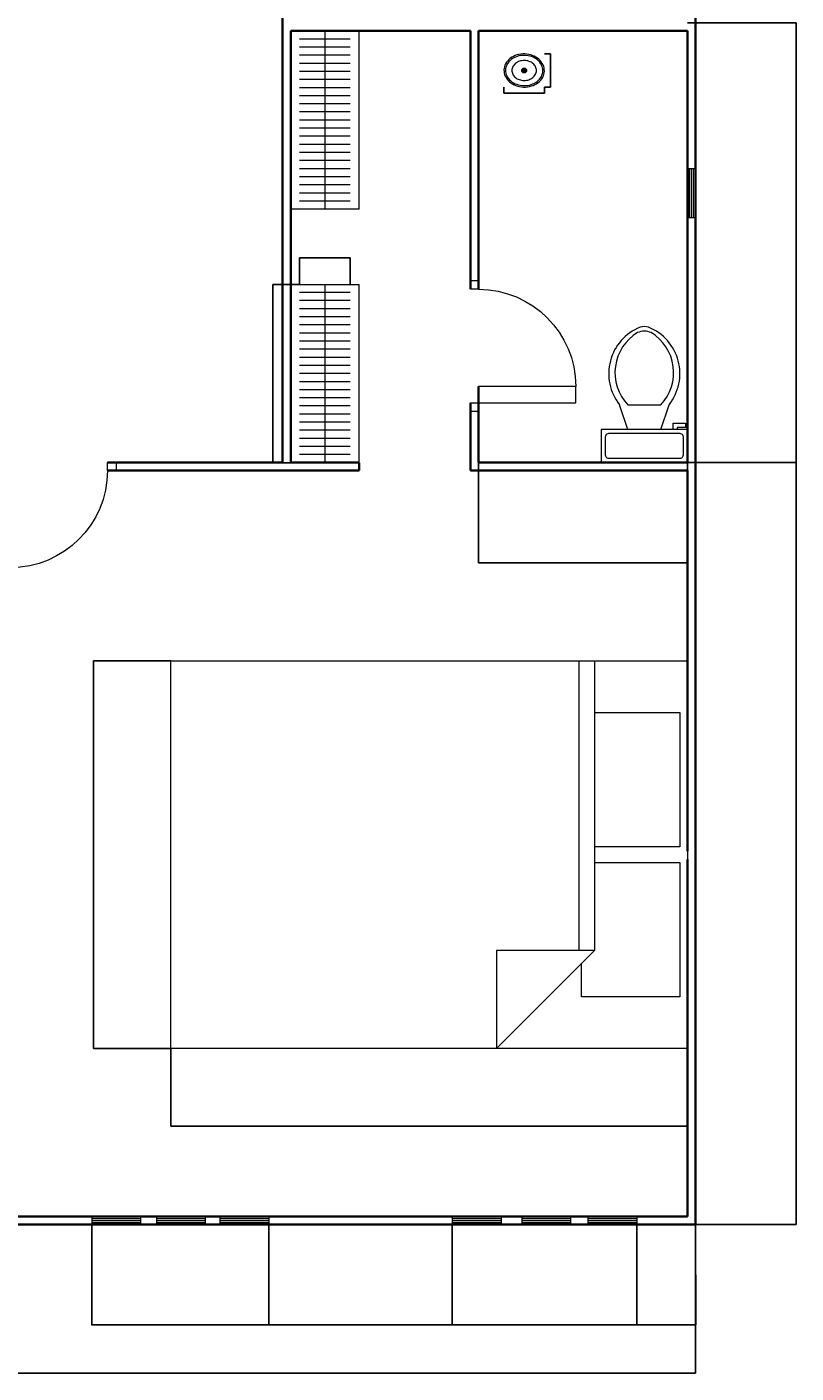
# Model space of a CAD drawing. Units: millimetres. Extents: x 1194 to 22780, y 83 to 13378.
# Tile 5 of 6: x 18030 to 22780, y 136 to 8443. Entities that reach past the tile are written whole.
import ezdxf

# ---------------------------------------------------------------- set-up
doc = ezdxf.new("R2010")
doc.units = ezdxf.units.MM
for name, color, linetype, lineweight in [('A-ANNO-DIMS', 2, 'Continuous', 18), ('A-DOOR', 3, 'Continuous', 18), ('A-FLOR-CASE', 8, 'Continuous', 13), ('A-FLOR-FIXT', 9, 'Continuous', 18), ('A-FURN', 8, 'Continuous', 18), ('A-GLAZ', 4, 'Continuous', 18), ('A-WALL', 7, 'Continuous', 35)]:
    doc.layers.add(name, color=color, linetype=linetype, lineweight=lineweight)
doc.styles.get("Standard").update_dxf_attribs({"font": 'arial.ttf'})
doc.dimstyles.get("Standard").update_dxf_attribs({"dimtxt": 0.18, "dimasz": 0.18, "dimexe": 0.18, "dimexo": 0.0625, "dimgap": 0.09, "dimtad": 0, "dimtih": 1, "dimtoh": 1, "dimdec": 4, "dimzin": 0, "dimdsep": 46, "dimtxsty": 'Standard', "dimcen": 0.09, "dimadec": 0, "dimazin": 0, "dimtfac": 1, "dimtdec": 4, "dimtofl": 0, "dimtmove": 0, "dimatfit": 3, "dimfxl": 1, "dimtolj": 1, "dimtzin": 0, "dimarcsym": 0})

# ---------------------------------------------------------------- blocks, each defined once
blk = doc.blocks.new('Bed - Queen')
for p, q in [((0, -80.00003), (0, 0)), ((0, 0), (59.99999, 0)), ((59.99999, 0), (59.99999, -80.00003)), ((7.99999, -1.2), (28.79998, -1.2)), ((7.99999, -14.4), (7.99999, -1.2)), ((28.79998, -1.2), (28.79998, -14.4)), ((31.19999, -1.2), (51.99999, -1.2)), ((31.19999, -14.4), (31.19999, -1.2)), ((51.99999, -1.2), (51.99999, -16.4)), ((0, -14.4), (44.8, -14.4)), ((59.99999, -29.6), (44.8, -14.4)), ((44.8, -14.4), (44.8, -29.6)), ((51.99999, -16.4), (46.79936, -16.4)), ((44.8, -16.8), (0, -16.8)), ((44.8, -29.6), (59.99999, -29.6)), ((59.99999, -80.00003), (0, -80.00003))]:
    blk.add_line(p, q)
blk = doc.blocks.new('Toilet - top')
for p, q in [((9.5, -6), (9.5, -2)), ((-10, -8.5), (-8, -8.5)), ((-10, -9.5), (-10, -8.5)), ((-7, -9.5), (-10, -9.5)), ((-8, -8.5), (-8, -8)), ((-7, -8), (-7, -9.5)), ((-4, -8), (-6, -14)), ((4, -8), (6, -14)), ((4, -14), (-4, -14))]:
    blk.add_line(p, q)
blk.add_lwpolyline([(10.5, -8), (10.5, 0), (-10.5, 0), (-10.5, -8)], close=True)
for points in [[(-9.5, -2), (-9.5, -6)], [(8.5, -1), (-8.5, -1)], [(-8.5, -7), (8.5, -7)]]:
    blk.add_lwpolyline(points)
for centre, radius, start, end in [((-8.62, -1.88), 0.884, 81.8699, 188.1301), ((8.62, -1.88), 0.884, 351.8699, 98.1301), ((-8.62, -6.12), 0.884, 171.8699, 278.1301), ((8.62, -6.12), 0.884, 261.8699, 8.1301), ((3.52, -21.58), 12.17, 141.4691, 247.9714), ((4.2, -21.82), 11.33, 136.3677, 238.9468), ((-3.52, -21.58), 12.17, 292.0284, 38.5307), ((-4.2, -21.82), 11.33, 301.053, 43.6321), ((0, -27.88), 4, 245.7318, 294.2682), ((0, -29), 4, 254.8605, 285.1395)]:
    blk.add_arc(centre, radius, start, end)
blk = doc.blocks.new('Sink - Oval top')
for p, q in [((-1, 0), (1, 0)), ((0, 1), (0, -1))]:
    blk.add_line(p, q)
for points in [[(-12.23, 0.39, 0.117634), (-11.46, -3.36, 0.104469), (-8.88, -6.8, 0.090016), (-5.08, -9.07, 0.08192), (-0.32, -10.02, 0.08192), (4.49, -9.38, 0.090016), (8.42, -7.36, 0.104469), (11.22, -4.09, 0.117634), (12.23, -0.39, 0.117634), (11.46, 3.36, 0.104469), (8.88, 6.8, 0.090016), (5.08, 9.07, 0.08192), (0.32, 10.02, 0.08192), (-4.49, 9.38, 0.090016), (-8.42, 7.36, 0.104469), (-11.22, 4.09, 0.117634)], [(-11.29, 0.16, 0.118622), (-10.52, -3.25, 0.104678), (-8.07, -6.36, 0.089562), (-4.54, -8.37, 0.081185), (-0.13, -9.15, 0.081185), (4.3, -8.49, 0.089562), (7.89, -6.58, 0.104678), (10.42, -3.55, 0.118622), (11.29, -0.16, 0.118622), (10.52, 3.25, 0.104678), (8.07, 6.36, 0.089562), (4.54, 8.37, 0.081185), (0.13, 9.15, 0.081185), (-4.3, 8.49, 0.089562), (-7.89, 6.58, 0.104678), (-10.42, 3.55, 0.118622)], [(-7.42, 0.08, 0.118283), (-6.91, -2.17, 0.104607), (-5.29, -4.21, 0.089718), (-2.97, -5.53, 0.081436), (-0.07, -6.04, 0.081436), (2.84, -5.59, 0.089718), (5.2, -4.33, 0.104607), (6.86, -2.32, 0.118283), (7.42, -0.08, 0.118283), (6.91, 2.17, 0.104607), (5.29, 4.21, 0.089718), (2.97, 5.53, 0.081436), (0.07, 6.04, 0.081436), (-2.84, 5.59, 0.089718), (-5.2, 4.33, 0.104607), (-6.86, 2.32, 0.118283)]]:
    blk.add_lwpolyline(points, format="xyb", close=True)
for radius in [1.5, 1]:
    blk.add_circle((0, 0), radius)
blk = doc.blocks.new('Window - Wood Frame 36 in. Wide plan')
for p, q in [((0, 6), (0, 0)), ((0, 4.5), (36, 4.5)), ((0, 3), (36, 3)), ((0, 1.5), (36, 1.5)), ((36, 6), (36, 0))]:
    blk.add_line(p, q)
blk = doc.blocks.new('DOOR-SWING-600')
for p, q in [((0, 0), (0, 600)), ((0, 600), (100, 600)), ((100, 600), (100, 0))]:
    blk.add_line(p, q)
blk.add_arc((100, 0), 600, 0, 90)
blk = doc.blocks.new('WARDROBE-RAIL-1100')
for p, q in [((156.2, 1100), (156.2, 0)), ((156.2, 1050), (0, 1050)), ((156.2, 1000), (0, 1000)), ((312.4, 1050), (156.2, 1050)), ((312.4, 1000), (156.2, 1000)), ((156.2, 950), (0, 950)), ((312.4, 950), (156.2, 950)), ((156.2, 900), (0, 900)), ((156.2, 850), (0, 850)), ((312.4, 900), (156.2, 900)), ((312.4, 850), (156.2, 850)), ((156.2, 800), (0, 800)), ((156.2, 750), (0, 750)), ((312.4, 800), (156.2, 800)), ((312.4, 750), (156.2, 750)), ((156.2, 700), (0, 700)), ((312.4, 700), (156.2, 700)), ((156.2, 650), (0, 650)), ((156.2, 600), (0, 600)), ((312.4, 650), (156.2, 650)), ((312.4, 600), (156.2, 600)), ((156.2, 550), (0, 550)), ((156.2, 500), (0, 500)), ((312.4, 550), (156.2, 550)), ((312.4, 500), (156.2, 500)), ((156.2, 450), (0, 450)), ((312.4, 450), (156.2, 450)), ((156.2, 400), (0, 400)), ((156.2, 350), (0, 350)), ((312.4, 400), (156.2, 400)), ((312.4, 350), (156.2, 350)), ((156.2, 300), (0, 300)), ((156.2, 250), (0, 250)), ((312.4, 300), (156.2, 300)), ((312.4, 250), (156.2, 250)), ((156.2, 200), (0, 200)), ((312.4, 200), (156.2, 200)), ((156.2, 150), (0, 150)), ((156.2, 100), (0, 100)), ((312.4, 150), (156.2, 150)), ((312.4, 100), (156.2, 100)), ((156.2, 50), (0, 50)), ((312.4, 50), (156.2, 50))]:
    blk.add_line(p, q)
blk = doc.blocks.new('*D23')
at = {"layer": 'A-ANNO-DIMS', "color": 0, "lineweight": -2, "transparency": 16777216}
for p, q in [((18919.4, 2138.4), (18919.4, 1659.8)), ((22109.2, 2138.4), (22109.2, 1659.8)), ((18919.6, 1659.9), (20513.7, 1659.9)), ((22109, 1659.9), (20515, 1659.9))]:
    blk.add_line(p, q, dxfattribs=at)
at = {"layer": 'A-ANNO-DIMS', "color": 0, "transparency": 16777216}
for points in [[(18919.6, 1660), (18919.6, 1659.9), (18919.4, 1659.9)], [(22109, 1660), (22109, 1659.9), (22109.2, 1659.9)]]:
    blk.add_solid(points, dxfattribs=at)
at = {"layer": 'Defpoints', "color": 0, "transparency": 16777216}
for p in [(18919.4, 2138.4), (22109.2, 2138.4), (22109.2, 1659.9)]:
    blk.add_point(p, dxfattribs=at)
at = {"layer": 'A-ANNO-DIMS', "color": 0, "transparency": 16777216, "insert": (20514.3, 1659.9), "char_height": 0.18, "attachment_point": 5}
blk.add_mtext('\\A1;BED 3190', dxfattribs=at)
blk = doc.blocks.new('*D24')
at = {"layer": 'A-ANNO-DIMS', "color": 0, "lineweight": -2, "transparency": 16777216}
for p, q in [((18919.3, 4530.8), (18440.7, 4530.8)), ((18440.9, 4530.6), (18440.9, 3334.8)), ((18440.9, 2138.6), (18440.9, 3334.4)), ((18919.3, 2138.4), (18440.7, 2138.4))]:
    blk.add_line(p, q, dxfattribs=at)
at = {"layer": 'A-ANNO-DIMS', "color": 0, "transparency": 16777216}
for points in [[(18440.9, 4530.6), (18441, 4530.6), (18440.9, 4530.8)], [(18440.9, 2138.6), (18441, 2138.6), (18440.9, 2138.4)]]:
    blk.add_solid(points, dxfattribs=at)
at = {"layer": 'Defpoints', "color": 0, "transparency": 16777216}
for p in [(18919.4, 4530.8), (18440.9, 2138.4), (18919.4, 2138.4)]:
    blk.add_point(p, dxfattribs=at)
at = {"layer": 'A-ANNO-DIMS', "color": 0, "transparency": 16777216, "insert": (18440.9, 3334.6), "char_height": 0.18, "attachment_point": 5}
blk.add_mtext('\\A1;2392', dxfattribs=at)
blk = doc.blocks.new('*D25')
at = {"layer": 'A-ANNO-DIMS', "color": 0, "lineweight": -2, "transparency": 16777216}
for p, q in [((20975.5, 8071.7), (20975.5, 8034)), ((21225.9, 8071.7), (21225.9, 8034)), ((20975.7, 8034.2), (21099.7, 8034.2)), ((21225.7, 8034.2), (21101.7, 8034.2))]:
    blk.add_line(p, q, dxfattribs=at)
at = {"layer": 'A-ANNO-DIMS', "color": 0, "transparency": 16777216}
for points in [[(20975.7, 8034.3), (20975.7, 8034.2), (20975.5, 8034.2)], [(21225.7, 8034.3), (21225.7, 8034.2), (21225.9, 8034.2)]]:
    blk.add_solid(points, dxfattribs=at)
at = {"layer": 'Defpoints', "color": 0, "transparency": 16777216}
for p in [(20975.5, 8071.8), (21225.9, 8071.8), (21225.9, 8034.2)]:
    blk.add_point(p, dxfattribs=at)
at = {"layer": 'A-ANNO-DIMS', "color": 0, "transparency": 16777216, "insert": (21100.7, 8034.2), "char_height": 0.18, "attachment_point": 5}
blk.add_mtext('\\A1;BASIN 250 TYP.', dxfattribs=at)
blk = doc.blocks.new('*D26')
at = {"layer": 'A-ANNO-DIMS', "color": 0, "lineweight": -2, "transparency": 16777216}
for p, q in [((21225.9, 8277.1), (21263.6, 8277.1)), ((21263.4, 8277), (21263.4, 8174.6)), ((21263.4, 8072), (21263.4, 8174.3)), ((21225.9, 8071.8), (21263.6, 8071.8))]:
    blk.add_line(p, q, dxfattribs=at)
at = {"layer": 'A-ANNO-DIMS', "color": 0, "transparency": 16777216}
for points in [[(21263.4, 8277), (21263.4, 8277), (21263.4, 8277.1)], [(21263.4, 8072), (21263.4, 8072), (21263.4, 8071.8)]]:
    blk.add_solid(points, dxfattribs=at)
at = {"layer": 'Defpoints', "color": 0, "transparency": 16777216}
for p in [(21225.9, 8277.1), (21263.4, 8277.1), (21225.9, 8071.8)]:
    blk.add_point(p, dxfattribs=at)
at = {"layer": 'A-ANNO-DIMS', "color": 0, "transparency": 16777216, "insert": (21263.4, 8174.5), "char_height": 0.18, "attachment_point": 5}
blk.add_mtext('\\A1;205 TYP.', dxfattribs=at)
blk = doc.blocks.new('*D41')
at = {"layer": 'A-ANNO-DIMS', "color": 0, "lineweight": -2, "transparency": 16777216}
for p, q in [((19714.1, 6854), (19549, 6854)), ((19549.2, 6853.8), (19549.2, 6304.2)), ((19549.2, 5754.2), (19549.2, 6303.8)), ((19714.1, 5754), (19549, 5754))]:
    blk.add_line(p, q, dxfattribs=at)
at = {"layer": 'A-ANNO-DIMS', "color": 0, "transparency": 16777216}
for points in [[(19549.2, 6853.8), (19549.2, 6853.8), (19549.2, 6854)], [(19549.2, 5754.2), (19549.2, 5754.2), (19549.2, 5754)]]:
    blk.add_solid(points, dxfattribs=at)
at = {"layer": 'Defpoints', "color": 0, "transparency": 16777216}
for p in [(19549.2, 6854), (19714.2, 6854), (19714.2, 5754)]:
    blk.add_point(p, dxfattribs=at)
at = {"layer": 'A-ANNO-DIMS', "color": 0, "transparency": 16777216, "insert": (19549.2, 6304), "char_height": 0.18, "attachment_point": 5}
blk.add_mtext('\\A1;CLOSET RAIL 1100 TYP.', dxfattribs=at)
blk = doc.blocks.new('*D42')
at = {"layer": 'A-ANNO-DIMS', "color": 0, "lineweight": -2, "transparency": 16777216}
for p, q in [((19714.2, 6854.1), (19714.2, 7019.2)), ((19714.4, 7019), (19869.8, 7019)), ((20026.4, 7019), (19871, 7019)), ((20026.6, 6854.1), (20026.6, 7019.2))]:
    blk.add_line(p, q, dxfattribs=at)
at = {"layer": 'A-ANNO-DIMS', "color": 0, "transparency": 16777216}
for points in [[(19714.4, 7019), (19714.4, 7019), (19714.2, 7019)], [(20026.4, 7019), (20026.4, 7019), (20026.6, 7019)]]:
    blk.add_solid(points, dxfattribs=at)
at = {"layer": 'Defpoints', "color": 0, "transparency": 16777216}
for p in [(20026.6, 7019), (19714.2, 6854), (20026.6, 6854)]:
    blk.add_point(p, dxfattribs=at)
at = {"layer": 'A-ANNO-DIMS', "color": 0, "transparency": 16777216, "insert": (19870.4, 7019), "char_height": 0.18, "attachment_point": 5}
blk.add_mtext('\\A1;312 TYP.', dxfattribs=at)
blk = doc.blocks.new('*D75')
at = {"layer": 'A-ANNO-DIMS', "color": 0, "lineweight": -2, "transparency": 16777216}
for p, q in [((22159.2, 1052.8), (22159.2, 135.6)), ((17634.2, 755.8), (17634.2, 135.6)), ((17634.4, 135.8), (19896.3, 135.8)), ((22159, 135.8), (19897.1, 135.8))]:
    blk.add_line(p, q, dxfattribs=at)
at = {"layer": 'A-ANNO-DIMS', "color": 0, "transparency": 16777216}
for points in [[(17634.4, 135.8), (17634.4, 135.8), (17634.2, 135.8)], [(22159, 135.8), (22159, 135.8), (22159.2, 135.8)]]:
    blk.add_solid(points, dxfattribs=at)
at = {"layer": 'Defpoints', "color": 0, "transparency": 16777216}
for p in [(22159.2, 1052.8), (17634.2, 755.8), (22159.2, 135.8)]:
    blk.add_point(p, dxfattribs=at)
at = {"layer": 'A-ANNO-DIMS', "color": 0, "transparency": 16777216, "insert": (19896.7, 135.8), "char_height": 0.18, "attachment_point": 5}
blk.add_mtext('\\A1;4525', dxfattribs=at)
blk = doc.blocks.new('*D76')
at = {"layer": 'A-ANNO-DIMS', "color": 0, "lineweight": -2, "transparency": 16777216}
for p, q in [((22109.3, 5755.8), (22779.4, 5755.8)), ((22779.2, 5755.6), (22779.2, 3404.5)), ((22779.2, 1053), (22779.2, 3404.1)), ((22159.3, 1052.8), (22779.4, 1052.8))]:
    blk.add_line(p, q, dxfattribs=at)
at = {"layer": 'A-ANNO-DIMS', "color": 0, "transparency": 16777216}
for points in [[(22779.2, 5755.6), (22779.2, 5755.6), (22779.2, 5755.8)], [(22779.2, 1053), (22779.2, 1053), (22779.2, 1052.8)]]:
    blk.add_solid(points, dxfattribs=at)
at = {"layer": 'Defpoints', "color": 0, "transparency": 16777216}
for p in [(22109.2, 5755.8), (22779.2, 5755.8), (22159.2, 1052.8)]:
    blk.add_point(p, dxfattribs=at)
at = {"layer": 'A-ANNO-DIMS', "color": 0, "transparency": 16777216, "insert": (22779.2, 3404.3), "char_height": 0.18, "attachment_point": 5}
blk.add_mtext('\\A1;4703', dxfattribs=at)
blk = doc.blocks.new('*D77')
at = {"layer": 'A-ANNO-DIMS', "color": 0, "lineweight": -2, "transparency": 16777216}
for p, q in [((22109.3, 8468.3), (22779.4, 8468.3)), ((22779.2, 8468.1), (22779.2, 7112.2)), ((22779.2, 5756), (22779.2, 7111.8)), ((22109.3, 5755.8), (22779.4, 5755.8))]:
    blk.add_line(p, q, dxfattribs=at)
at = {"layer": 'A-ANNO-DIMS', "color": 0, "transparency": 16777216}
for points in [[(22779.2, 8468.1), (22779.2, 8468.1), (22779.2, 8468.3)], [(22779.2, 5756), (22779.2, 5756), (22779.2, 5755.8)]]:
    blk.add_solid(points, dxfattribs=at)
at = {"layer": 'Defpoints', "color": 0, "transparency": 16777216}
for p in [(22109.2, 8468.3), (22779.2, 8468.3), (22109.2, 5755.8)]:
    blk.add_point(p, dxfattribs=at)
at = {"layer": 'A-ANNO-DIMS', "color": 0, "transparency": 16777216, "insert": (22779.2, 7112), "char_height": 0.18, "attachment_point": 5}
blk.add_mtext('\\A1;2712.5', dxfattribs=at)
blk = doc.blocks.new('*D85')
at = {"layer": 'A-ANNO-DIMS', "color": 0, "lineweight": -2, "transparency": 16777216}
for p, q in [((20818.9, 5755.7), (20818.9, 5135.6)), ((22109.2, 5755.7), (22109.2, 5135.6)), ((20819.1, 5135.8), (21463.6, 5135.8)), ((22109, 5135.8), (21464.5, 5135.8))]:
    blk.add_line(p, q, dxfattribs=at)
at = {"layer": 'A-ANNO-DIMS', "color": 0, "transparency": 16777216}
for points in [[(20819.1, 5135.8), (20819.1, 5135.7), (20818.9, 5135.8)], [(22109, 5135.8), (22109, 5135.7), (22109.2, 5135.8)]]:
    blk.add_solid(points, dxfattribs=at)
at = {"layer": 'Defpoints', "color": 0, "transparency": 16777216}
for p in [(20818.9, 5755.8), (22109.2, 5755.8), (20818.9, 5135.8)]:
    blk.add_point(p, dxfattribs=at)
at = {"layer": 'A-ANNO-DIMS', "color": 0, "transparency": 16777216, "insert": (21464.1, 5135.8), "char_height": 0.18, "attachment_point": 5}
blk.add_mtext('\\A1;1290.3', dxfattribs=at)
blk = doc.blocks.new('*D89')
at = {"layer": 'A-ANNO-DIMS', "color": 0, "lineweight": -2, "transparency": 16777216}
for p, q in [((18430.4, 1052.4), (18430.4, 432.3)), ((19524.1, 1052.4), (19524.1, 432.3)), ((18430.6, 432.5), (18976.8, 432.5)), ((19523.9, 432.5), (18977.7, 432.5))]:
    blk.add_line(p, q, dxfattribs=at)
at = {"layer": 'A-ANNO-DIMS', "color": 0, "transparency": 16777216}
for points in [[(18430.6, 432.5), (18430.6, 432.5), (18430.4, 432.5)], [(19523.9, 432.5), (19523.9, 432.5), (19524.1, 432.5)]]:
    blk.add_solid(points, dxfattribs=at)
at = {"layer": 'Defpoints', "color": 0, "transparency": 16777216}
for p in [(18430.4, 1052.5), (19524.1, 1052.5), (18430.4, 432.5)]:
    blk.add_point(p, dxfattribs=at)
at = {"layer": 'A-ANNO-DIMS', "color": 0, "transparency": 16777216, "insert": (18977.2, 432.5), "char_height": 0.18, "attachment_point": 5}
blk.add_mtext('\\A1;1093.6', dxfattribs=at)
blk = doc.blocks.new('*D90')
at = {"layer": 'A-ANNO-DIMS', "color": 0, "lineweight": -2, "transparency": 16777216}
for p, q in [((19524.1, 1052.4), (19524.1, 432.3)), ((20656, 1052.4), (20656, 432.3)), ((19524.2, 432.5), (20089.7, 432.5)), ((20655.9, 432.5), (20090.4, 432.5))]:
    blk.add_line(p, q, dxfattribs=at)
at = {"layer": 'A-ANNO-DIMS', "color": 0, "transparency": 16777216}
for points in [[(19524.2, 432.5), (19524.2, 432.5), (19524.1, 432.5)], [(20655.9, 432.5), (20655.9, 432.5), (20656, 432.5)]]:
    blk.add_solid(points, dxfattribs=at)
at = {"layer": 'Defpoints', "color": 0, "transparency": 16777216}
for p in [(19524.1, 1052.5), (20656, 1052.5), (19524.1, 432.5)]:
    blk.add_point(p, dxfattribs=at)
at = {"layer": 'A-ANNO-DIMS', "color": 0, "transparency": 16777216, "insert": (20090.1, 432.5), "char_height": 0.18, "attachment_point": 5}
blk.add_mtext('\\A1;1132', dxfattribs=at)
blk = doc.blocks.new('*D91')
at = {"layer": 'A-ANNO-DIMS', "color": 0, "lineweight": -2, "transparency": 16777216}
for p, q in [((20656, 1052.4), (20656, 432.3)), ((21795.9, 1052.4), (21795.9, 432.3)), ((20656.2, 432.5), (21225.5, 432.5)), ((21795.7, 432.5), (21226.4, 432.5))]:
    blk.add_line(p, q, dxfattribs=at)
at = {"layer": 'A-ANNO-DIMS', "color": 0, "transparency": 16777216}
for points in [[(20656.2, 432.5), (20656.2, 432.5), (20656, 432.5)], [(21795.7, 432.5), (21795.7, 432.5), (21795.9, 432.5)]]:
    blk.add_solid(points, dxfattribs=at)
at = {"layer": 'Defpoints', "color": 0, "transparency": 16777216}
for p in [(20656, 1052.5), (21795.9, 1052.5), (20656, 432.5)]:
    blk.add_point(p, dxfattribs=at)
at = {"layer": 'A-ANNO-DIMS', "color": 0, "transparency": 16777216, "insert": (21226, 432.5), "char_height": 0.18, "attachment_point": 5}
blk.add_mtext('\\A1;1139.8', dxfattribs=at)
blk = doc.blocks.new('*D92')
at = {"layer": 'A-ANNO-DIMS', "color": 0, "lineweight": -2, "transparency": 16777216}
for p, q in [((21795.9, 1052.4), (21796.4, 432.3)), ((22159.2, 1052.8), (22159.8, 432.6)), ((21796.6, 432.5), (21977.6, 432.6)), ((22159.6, 432.8), (21978.6, 432.6))]:
    blk.add_line(p, q, dxfattribs=at)
at = {"layer": 'A-ANNO-DIMS', "color": 0, "transparency": 16777216}
for points in [[(21796.6, 432.5), (21796.6, 432.5), (21796.4, 432.5)], [(22159.6, 432.8), (22159.6, 432.8), (22159.8, 432.8)]]:
    blk.add_solid(points, dxfattribs=at)
at = {"layer": 'Defpoints', "color": 0, "transparency": 16777216}
for p in [(21795.9, 1052.5), (22159.2, 1052.8), (21796.4, 432.5)]:
    blk.add_point(p, dxfattribs=at)
at = {"layer": 'A-ANNO-DIMS', "color": 0, "transparency": 16777216, "insert": (21978.1, 432.6), "char_height": 0.18, "attachment_point": 5}
blk.add_mtext('\\A1;363.36', dxfattribs=at)

msp = doc.modelspace()

# ---------------------------------------------------------------- linework, layer by layer
at = {"layer": 'A-DOOR'}
for p, q in [((20768.943, 6823.977), (20768.943, 6877.662)), ((20768.943, 6877.662), (20818.943, 6877.662)), ((20818.943, 6823.977), (20768.943, 6823.977)), ((20818.943, 6877.662), (20818.943, 6823.977)), ((20818.943, 6070.293), (20818.943, 6223.977)), ((20768.943, 6070.293), (20768.943, 6123.977)), ((20768.943, 6123.977), (20818.943, 6123.977)), ((20818.943, 6070.293), (20768.943, 6070.293)), ((18527.474, 5705.774), (18527.474, 5755.774)), ((18527.474, 5755.774), (18581.159, 5755.774)), ((18581.159, 5755.774), (18581.159, 5705.774)), ((18581.159, 5755.774), (18581.159, 5705.774)), ((18581.159, 5705.774), (18527.474, 5705.774))]:
    msp.add_line(p, q, dxfattribs=at)
at = {"layer": 'A-FLOR-CASE'}
for p, q in [((19659.207, 8418.274), (19659.207, 6968.274)), ((20081.574, 8418.274), (19659.207, 8418.274)), ((19870.39, 8418.274), (19714.184, 8418.274)), ((20026.596, 8418.274), (19870.39, 8418.274)), ((20081.574, 7318.714), (20081.574, 8418.274)), ((19659.207, 7318.714), (19659.207, 5868.714)), ((20081.574, 7318.714), (19659.207, 7318.714)), ((19870.39, 7318.714), (19714.184, 7318.714)), ((19870.39, 7318.274), (19714.184, 7318.274)), ((19870.39, 7318.714), (19870.39, 7318.274)), ((20026.596, 7318.714), (19870.39, 7318.714)), ((20026.596, 7318.274), (19870.39, 7318.274)), ((19659.207, 6853.564), (20081.574, 6853.564)), ((20081.574, 5754.003), (20081.574, 6853.564)), ((19659.207, 5754.003), (20081.574, 5754.003))]:
    msp.add_line(p, q, dxfattribs=at)
at = {"layer": 'A-WALL'}
for p, q in [((22159.207, 1052.813), (22159.207, 12730.774)), ((19609.207, 8608.432), (19609.207, 8142.853)), ((19609.207, 8418.274), (19609.207, 6618.274)), ((20309.207, 8418.274), (19659.207, 8418.274)), ((19659.207, 8418.274), (19659.207, 6668.274)), ((19659.207, 8192.853), (19659.207, 8418.274)), ((20768.943, 8418.274), (20309.207, 8418.274)), ((20768.943, 8418.274), (20768.943, 6823.977)), ((20768.943, 6823.977), (20768.943, 8418.274)), ((22109.207, 8418.274), (20818.943, 8418.274)), ((20818.943, 8418.274), (20818.943, 6823.977)), ((22109.207, 8418.274), (22109.207, 6930.774)), ((22109.207, 6930.774), (22109.207, 6668.274)), ((19659.207, 6668.274), (19659.207, 6618.274)), ((22109.207, 6668.274), (22109.207, 6618.274)), ((19609.207, 6618.274), (19609.207, 5755.774)), ((19659.207, 6618.274), (19659.207, 5755.774)), ((22109.207, 6618.274), (22109.207, 5755.774)), ((20818.943, 6223.977), (20818.943, 5755.774)), ((20768.943, 5755.774), (20768.943, 6123.977)), ((18527.474, 5755.774), (19609.207, 5755.774)), ((19659.207, 5755.774), (20081.574, 5755.774)), ((20081.574, 5754.003), (20081.574, 5705.774)), ((20768.943, 5755.774), (20768.943, 5705.774)), ((20818.943, 5755.774), (22109.207, 5755.774)), ((18527.474, 5705.774), (20081.574, 5705.774)), ((20768.943, 5705.774), (22109.207, 5705.774)), ((22109.207, 5705.774), (22109.207, 3355.774)), ((22109.207, 3305.774), (22109.207, 1805.774)), ((22109.207, 1102.813), (22109.207, 3305.774)), ((17634.207, 1102.813), (22109.207, 1102.813)), ((17584.207, 1052.813), (22159.207, 1052.813))]:
    msp.add_line(p, q, dxfattribs=at)

# ---------------------------------------------------------------- block references
at = {"layer": 'A-DOOR', "extrusion": (0, 0, -1), "zscale": -1}
for p, rotation in [((-20818.943, 6123.978), 90.00000000000011), ((-17827.475, 5705.774), 180)]:
    msp.add_blockref('DOOR-SWING-600', p, dxfattribs=dict(at, rotation=rotation))
at = {"layer": 'A-FLOR-CASE'}
for p in [(19714.184, 7318.274), (19714.184, 5754.004)]:
    msp.add_blockref('WARDROBE-RAIL-1100', p, dxfattribs=at)
at = {"layer": 'A-FLOR-FIXT', "xscale": 10.19841034025665, "yscale": 10.19841034025665, "zscale": 10.19841034025665}
msp.add_blockref('Sink - Oval top', (21100.669, 8174.467), dxfattribs=at)
at = {"layer": 'A-FLOR-FIXT', "xscale": 25.4, "yscale": 25.4, "zscale": 25.4, "rotation": 180}
msp.add_blockref('Toilet - top', (21842.507, 5755.774), dxfattribs=at)
at = {"layer": 'A-FURN', "xscale": 39.87258705656031, "yscale": 39.87258705656031, "zscale": 39.87258705656031, "rotation": 270}
msp.add_blockref('Bed - Queen', (22109.207, 4530.774), dxfattribs=at)
at = {"layer": 'A-GLAZ', "xscale": 8.388003104210137, "yscale": 8.388003104210137, "zscale": 8.388003104210137, "rotation": 90}
msp.add_blockref('Window - Wood Frame 36 in. Wide plan', (22159.207, 7266.783), dxfattribs=at)
at = {"layer": 'A-GLAZ', "xscale": 8.388003104210137, "yscale": 8.388003104210137, "zscale": 8.388003104210137}
for p in [(18430.442, 1052.485), (18829.534, 1052.485), (19222.084, 1052.485), (20656.05, 1052.485), (21085.439, 1052.485), (21493.882, 1052.485)]:
    msp.add_blockref('Window - Wood Frame 36 in. Wide plan', p, dxfattribs=at)

# ---------------------------------------------------------------- dimensions: what is measured, and where the dimension line sits
at = {"layer": 'A-ANNO-DIMS'}
for base, p1, p2, angle, override, picture, middle in [((22779.207, 8468.274), (22109.207, 5755.774), (22109.207, 8468.274), 90, {"dimdec": 1, "dimlfac": 1, "dimrnd": 0, "dimzin": 0, "dimdsep": 46, "dimlunit": 2}, '*D77', (22779.207, 7112.024)), ((20818.943, 5135.774), (22109.207, 5755.774), (20818.943, 5755.774), 180, {"dimdec": 1, "dimlfac": 1, "dimrnd": 0, "dimzin": 0, "dimdsep": 46, "dimlunit": 2}, '*D85', (21464.075, 5135.774)), ((22779.207, 5755.774), (22159.207, 1052.813), (22109.207, 5755.774), 90, {"dimdec": 0, "dimlfac": 1, "dimrnd": 0, "dimzin": 0, "dimdsep": 46, "dimlunit": 2}, '*D76', (22779.207, 3404.293)), ((18440.927, 2138.419), (18919.398, 4530.774), (18919.398, 2138.419), 270, {"dimdec": 0, "dimlfac": 1, "dimrnd": 0, "dimzin": 0, "dimdsep": 46, "dimlunit": 2}, '*D24', (18440.927, 3334.596)), ((18430.442, 432.485), (19524.052, 1052.485), (18430.442, 1052.485), 180, {"dimdec": 1, "dimlfac": 1, "dimrnd": 0, "dimzin": 0, "dimdsep": 46, "dimlunit": 2}, '*D89', (18977.247, 432.485)), ((19524.052, 432.485), (20656.05, 1052.485), (19524.052, 1052.485), 180, {"dimdec": 0, "dimlfac": 1, "dimrnd": 0, "dimzin": 0, "dimdsep": 46, "dimlunit": 2}, '*D90', (20090.051, 432.485)), ((20656.05, 432.485), (21795.851, 1052.485), (20656.05, 1052.485), 180, {"dimdec": 1, "dimlfac": 1, "dimrnd": 0, "dimzin": 0, "dimdsep": 46, "dimlunit": 2}, '*D91', (21225.95, 432.485)), ((21796.41, 432.485), (22159.207, 1052.813), (21795.851, 1052.485), 180.0517236, {"dimdec": 2, "dimlfac": 1, "dimrnd": 0, "dimzin": 0, "dimdsep": 46, "dimlunit": 2}, '*D92', (21978.088, 432.649))]:
    dim = msp.add_linear_dim(base=base, p1=p1, p2=p2, angle=angle, dimstyle='Standard', override=override, dxfattribs=at)
    dim.commit()
    dim.dimension.update_dxf_attribs({"geometry": picture, "text_midpoint": middle})
for base, p1, p2, text, picture, middle in [((21263.416, 8277.147), (21225.859, 8071.786), (21225.859, 8277.147), '<> TYP.', '*D26', (21263.416, 8174.467)), ((19549.184, 6854.003), (19714.184, 5754.003), (19714.184, 6854.003), 'CLOSET RAIL <> TYP.', '*D41', (19549.184, 6304.003))]:
    dim = msp.add_linear_dim(base=base, p1=p1, p2=p2, angle=90, text=text, dimstyle='Standard', override={"dimdec": 0, "dimlfac": 1, "dimrnd": 0, "dimzin": 0, "dimdsep": 46, "dimlunit": 2}, dxfattribs=at)
    dim.commit()
    dim.dimension.update_dxf_attribs({"geometry": picture, "text_midpoint": middle})
for base, p1, p2, text, picture, middle in [((21225.859, 8034.229), (20975.479, 8071.786), (21225.859, 8071.786), 'BASIN <> TYP.', '*D25', (21100.669, 8034.229)), ((20026.596, 7019.003), (19714.184, 6854.003), (20026.596, 6854.003), '<> TYP.', '*D42', (19870.39, 7019.003)), ((22109.207, 1659.948), (18919.398, 2138.419), (22109.207, 2138.419), 'BED <>', '*D23', (20514.303, 1659.948))]:
    dim = msp.add_linear_dim(base=base, p1=p1, p2=p2, text=text, dimstyle='Standard', override={"dimdec": 0, "dimlfac": 1, "dimrnd": 0, "dimzin": 0, "dimdsep": 46, "dimlunit": 2}, dxfattribs=at)
    dim.commit()
    dim.dimension.update_dxf_attribs({"geometry": picture, "text_midpoint": middle})
dim = msp.add_linear_dim(base=(22159.207, 135.817), p1=(17634.207, 755.817), p2=(22159.207, 1052.813), dimstyle='Standard', override={"dimdec": 0, "dimlfac": 1, "dimrnd": 0, "dimzin": 0, "dimdsep": 46, "dimlunit": 2}, dxfattribs=at)
dim.commit()
dim.dimension.update_dxf_attribs({"geometry": '*D75', "text_midpoint": (19896.707, 135.817)})

doc.saveas('drawing.dxf')
